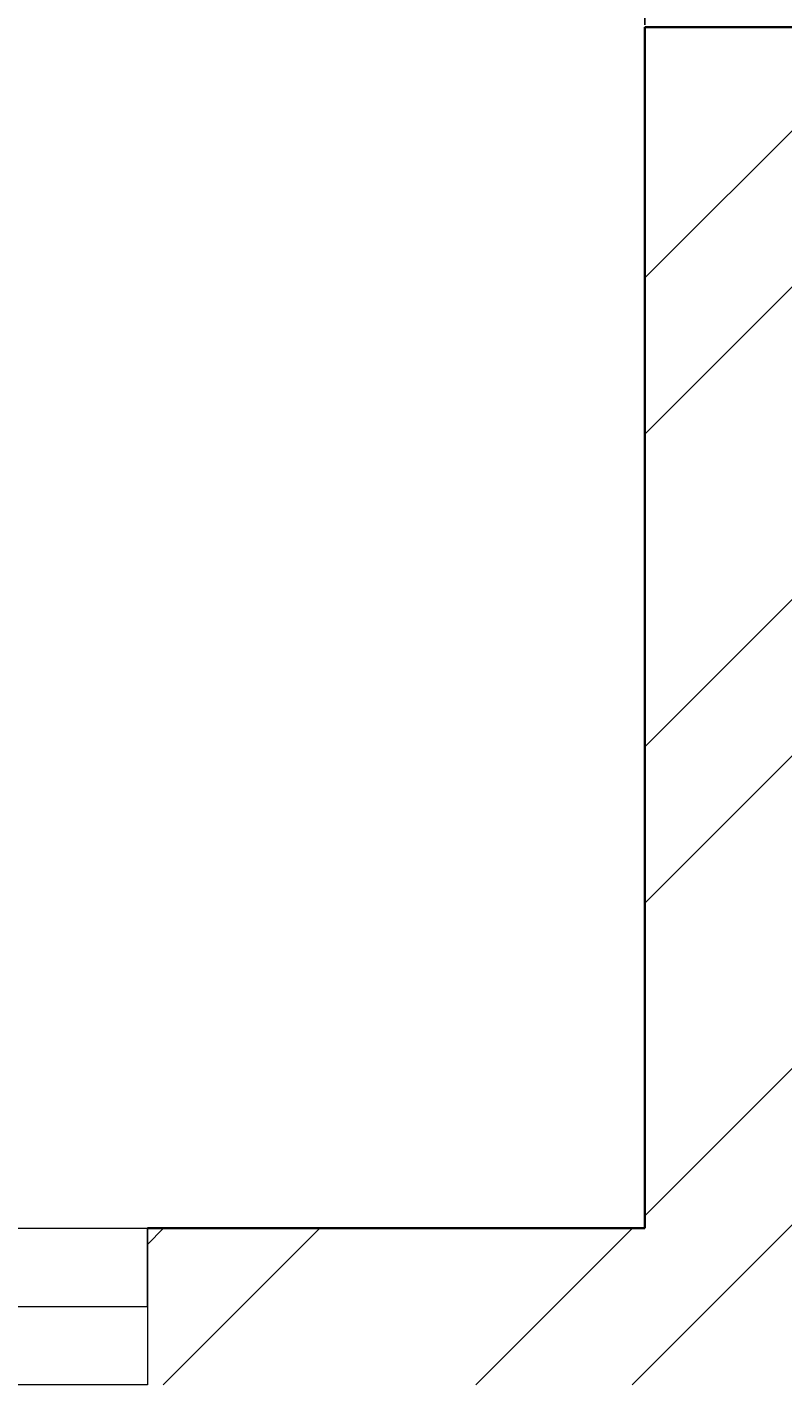
# Model space of a CAD drawing. Units: inches. Extents: x 1885 to 2748, y 783 to 2421.
# Tile 95 of 117: x 2341 to 2363, y 2314 to 2353. Entities that reach past the tile are written whole.
import ezdxf

# ---------------------------------------------------------------- set-up
doc = ezdxf.new("R2010")
doc.units = ezdxf.units.IN
for name, color, linetype, lineweight in [('A-ANNO-DIMS', 2, 'Continuous', 18), ('A-GLAZ', 181, 'Continuous', 18), ('A-WALL', 7, 'Continuous', 35)]:
    doc.layers.add(name, color=color, linetype=linetype, lineweight=lineweight)
doc.layers.add('A-WALL-PATT', color=85, linetype='Continuous', lineweight=13, true_color=0x58ba48)
doc.styles.get("Standard").update_dxf_attribs({"font": 'arial.ttf'})
doc.dimstyles.get("Standard").update_dxf_attribs({"dimtxt": 0.18, "dimasz": 0.18, "dimexe": 0.18, "dimexo": 0.0625, "dimgap": 0.09, "dimtad": 0, "dimtih": 1, "dimtoh": 1, "dimdec": 4, "dimzin": 0, "dimdsep": 46, "dimtxsty": 'Standard', "dimcen": 0.09, "dimadec": 0, "dimazin": 0, "dimtfac": 1, "dimtdec": 4, "dimtofl": 0, "dimtmove": 0, "dimatfit": 3, "dimfxl": 1, "dimtolj": 1, "dimtzin": 0, "dimarcsym": 0})

# ---------------------------------------------------------------- blocks, each defined once
blk = doc.blocks.new('WIN-24')
for p, q in [((0.001, 4.496), (0.001, -0.004)), ((0.001, 4.496), (24.001, 4.496)), ((24.001, 2.246), (24.001, 4.496)), ((24.001, 4.496), (24.001, -0.004)), ((0.001, -0.004), (0.001, 2.246)), ((0.001, 2.246), (24.001, 2.246)), ((24.001, -0.004), (0.001, -0.004))]:
    blk.add_line(p, q)
blk = doc.blocks.new('*D52')
at = {"layer": 'A-ANNO-DIMS', "color": 0, "lineweight": -2, "transparency": 16777216}
for p, q in [((2310.774, 2348.068), (2310.774, 2420.936)), ((2310.954, 2420.756), (2334.551, 2420.756)), ((2358.594, 2420.756), (2334.996, 2420.756)), ((2358.774, 2352.568), (2358.774, 2420.936))]:
    blk.add_line(p, q, dxfattribs=at)
at = {"layer": 'A-ANNO-DIMS', "color": 0, "transparency": 16777216}
for points in [[(2310.954, 2420.786), (2310.954, 2420.726), (2310.774, 2420.756)], [(2358.594, 2420.786), (2358.594, 2420.726), (2358.774, 2420.756)]]:
    blk.add_solid(points, dxfattribs=at)
at = {"layer": 'Defpoints', "color": 0, "transparency": 16777216}
for p in [(2358.774, 2420.756), (2358.774, 2352.506), (2310.774, 2348.006)]:
    blk.add_point(p, dxfattribs=at)
at = {"layer": 'A-ANNO-DIMS', "color": 0, "transparency": 16777216, "insert": (2334.774, 2420.756), "char_height": 0.18, "attachment_point": 5}
blk.add_mtext('\\A1;48', dxfattribs=at)

msp = doc.modelspace()

# ---------------------------------------------------------------- hatches: boundary and pattern name
at = {"layer": 'A-WALL-PATT'}
h = msp.add_hatch(dxfattribs=at)
h.set_pattern_fill('ANSI32', color=256)
h.paths.add_polyline_path([(2007.772, 2318.006), (1980.774, 2318.006), (1980.774, 2281.215), (1985.274, 2281.215), (1985.274, 2313.506), (2007.772, 2313.506), (2007.772, 2315.756)])
h.paths.add_polyline_path([(2094.324, 2318.006), (2067.772, 2318.006), (2067.772, 2313.506), (2094.324, 2313.506), (2094.324, 2315.756)])
h.paths.add_polyline_path([(2131.367, 2315.756), (2131.367, 2318.006), (2131.189, 2318.006), (2112.609, 2318.006), (2112.609, 2313.506), (2117.274, 2313.506), (2117.274, 2255.201), (2121.774, 2255.201), (2121.774, 2313.506), (2131.367, 2313.506)])
h.paths.add_polyline_path([(2190.512, 2318.006), (2155.367, 2318.006), (2155.367, 2313.506), (2169.774, 2313.506), (2169.774, 2229.506), (2121.774, 2229.506), (2121.774, 2233.451), (2119.524, 2233.451), (2117.274, 2233.451), (2117.274, 2201.101), (2121.774, 2201.101), (2121.774, 2225.006), (2169.774, 2225.006), (2169.774, 2165.006), (2306.274, 2165.006), (2306.274, 2066.006), (2310.774, 2066.006), (2344.274, 2066.006), (2486.274, 2066.006), (2486.274, 1886.006), (2483.02, 1886.006), (2483.02, 1881.506), (2486.274, 1881.506), (2486.274, 1880.678), (2490.774, 1880.678), (2490.774, 2070.506), (2344.274, 2070.506), (2310.774, 2070.506), (2310.774, 2165.006), (2310.774, 2173.636), (2308.524, 2173.636), (2306.274, 2173.636), (2306.274, 2169.506), (2174.274, 2169.506), (2174.274, 2313.506), (2190.512, 2313.506), (2190.512, 2315.756)])
h.paths.add_polyline_path([(1985.274, 2221.215), (1980.774, 2221.215), (1980.774, 2165.006), (1992.774, 2165.006), (1992.774, 2141.927), (1997.274, 2141.927), (1997.274, 2165.006), (2117.274, 2165.006), (2117.274, 2163.126), (2121.774, 2163.126), (2121.774, 2172.734), (2119.524, 2172.734), (2117.274, 2172.734), (2117.274, 2169.506), (1985.274, 2169.506)])
h.paths.add_polyline_path([(1997.274, 2105.927), (1992.774, 2105.927), (1992.774, 2070.506), (2016.774, 2070.506), (2016.774, 2059.123), (2019.024, 2059.123), (2021.274, 2059.123), (2021.274, 2070.506), (2117.274, 2070.506), (2117.274, 2022.506), (2114.423, 2022.506), (2114.423, 2018.006), (2123.627, 2018.006), (2123.627, 2020.256), (2123.627, 2022.506), (2121.774, 2022.506), (2121.774, 2142.587), (2119.524, 2142.587), (2117.274, 2142.587), (2117.274, 2075.006), (1997.274, 2075.006)])
h.paths.add_polyline_path([(2092.029, 2020.256), (2092.029, 2022.506), (2021.274, 2022.506), (2021.274, 2035.123), (2016.774, 2035.123), (2016.774, 2018.006), (2016.774, 1978.784), (2021.274, 1978.784), (2021.274, 2018.006), (2092.029, 2018.006)])
h.paths.add_polyline_path([(2260.938, 2022.506), (2153.105, 2022.506), (2153.105, 2020.256), (2153.105, 2018.006), (2155.274, 2018.006), (2155.274, 1886.006), (2107.629, 1886.006), (2107.629, 1881.506), (2182.911, 1881.506), (2182.911, 1883.756), (2182.911, 1886.006), (2159.774, 1886.006), (2159.774, 2018.006), (2260.938, 2018.006), (2260.938, 2020.256)])
h.paths.add_polyline_path([(2047.629, 1883.756), (2047.629, 1886.006), (2021.274, 1886.006), (2021.274, 1918.784), (2019.024, 1918.784), (2016.774, 1918.784), (2016.774, 1881.506), (2047.629, 1881.506)])
h.paths.add_polyline_path([(2306.361, 1883.756), (2306.361, 1886.006), (2296.274, 1886.006), (2296.274, 1982.006), (2316.535, 1982.006), (2316.535, 1984.256), (2316.535, 1986.506), (2296.274, 1986.506), (2296.274, 2022.506), (2289.276, 2022.506), (2289.276, 2018.006), (2291.774, 2018.006), (2291.774, 1886.006), (2242.911, 1886.006), (2242.911, 1881.506), (2306.361, 1881.506)], flags=17)
h.paths.add_polyline_path([(1985.274, 1843.006), (2021.6, 1843.006), (2021.534, 1845.441), (2021.477, 1847.506), (1980.774, 1847.506), (1980.774, 1809.446), (1985.274, 1809.446)])
h.paths.add_polyline_path([(2131.482, 1845.256), (2131.482, 1847.506), (2081.534, 1847.506), (2081.534, 1843.006), (2117.274, 1843.006), (2117.274, 1784.147), (2119.524, 1784.147), (2121.774, 1784.147), (2121.774, 1843.006), (2131.482, 1843.006)])
h.paths.add_polyline_path([(2203.886, 1847.506), (2155.482, 1847.506), (2155.482, 1843.006), (2169.774, 1843.006), (2169.774, 1759.006), (2121.774, 1759.006), (2121.774, 1761.457), (2117.274, 1761.457), (2117.274, 1730.429), (2121.774, 1730.429), (2121.774, 1754.506), (2177.421, 1754.506), (2177.421, 1756.756), (2177.421, 1759.006), (2174.274, 1759.006), (2174.274, 1843.006), (2203.886, 1843.006)])
h.paths.add_polyline_path([(2335.554, 1845.256), (2335.554, 1847.506), (2239.886, 1847.506), (2239.886, 1843.006), (2306.274, 1843.006), (2306.274, 1759.006), (2199.486, 1759.006), (2199.486, 1754.506), (2310.774, 1754.506), (2310.774, 1843.006), (2335.554, 1843.006)])
h.paths.add_polyline_path([(2348.774, 2022.506), (2344.274, 2022.506), (2344.274, 1986.506), (2341.681, 1986.506), (2341.681, 1982.006), (2344.274, 1982.006), (2344.274, 1886.006), (2330.361, 1886.006), (2330.361, 1881.506), (2361.627, 1881.506), (2361.627, 1883.756), (2361.627, 1886.006), (2348.774, 1886.006)], flags=17)
h.paths.add_polyline_path([(2283.251, 2315.756), (2283.251, 2318.006), (2238.512, 2318.006), (2238.512, 2313.506), (2283.251, 2313.506)], flags=17)
h.paths.add_polyline_path([(2363.274, 2348.006), (2388.677, 2348.006), (2388.677, 2350.256), (2388.677, 2352.506), (2358.774, 2352.506), (2358.774, 2348.006), (2358.774, 2318.006), (2344.481, 2318.006), (2344.481, 2313.506), (2358.774, 2313.506), (2358.774, 2229.506), (2310.774, 2229.506), (2310.774, 2231.952), (2306.274, 2231.952), (2306.274, 2205.611), (2310.774, 2205.611), (2310.774, 2225.006), (2358.774, 2225.006), (2358.774, 2211.506), (2452.329, 2211.506), (2452.329, 2213.756), (2452.329, 2216.006), (2363.274, 2216.006), (2363.274, 2318.006)])
h.paths.add_polyline_path([(2310.774, 2313.506), (2320.481, 2313.506), (2320.481, 2315.756), (2320.481, 2318.006), (2302.728, 2318.006), (2302.728, 2313.506), (2306.274, 2313.506), (2306.274, 2251.076), (2310.774, 2251.076)], flags=17)
h.paths.add_polyline_path([(2490.774, 2352.506), (2486.274, 2352.506), (2448.677, 2352.506), (2448.677, 2348.006), (2486.274, 2348.006), (2486.274, 2318.006), (2486.274, 2216.006), (2481.78, 2216.006), (2481.78, 2211.506), (2486.274, 2211.506), (2486.274, 2165.006), (2493.289, 2165.006), (2493.289, 2167.256), (2493.289, 2169.506), (2490.774, 2169.506), (2490.774, 2313.506), (2494.429, 2313.506), (2494.429, 2318.006), (2490.774, 2318.006)])
h.paths.add_polyline_path([(2534.653, 2318.006), (2515.691, 2318.006), (2515.691, 2313.506), (2534.653, 2313.506), (2534.653, 2315.756)])
h.paths.add_polyline_path([(2618.274, 2318.006), (2594.653, 2318.006), (2594.653, 2313.506), (2613.774, 2313.506), (2613.774, 2281.706), (2618.274, 2281.706)])
h.paths.add_polyline_path([(2618.274, 2221.706), (2613.774, 2221.706), (2613.774, 2169.506), (2554.019, 2169.506), (2554.019, 2165.006), (2613.774, 2165.006), (2613.774, 2152.878), (2618.274, 2152.878)])
h.paths.add_polyline_path([(2618.274, 2128.878), (2616.024, 2128.878), (2613.774, 2128.878), (2613.774, 2117.006), (2529.774, 2117.006), (2529.774, 2165.006), (2532.848, 2165.006), (2532.848, 2169.506), (2522.867, 2169.506), (2522.867, 2165.006), (2525.274, 2165.006), (2525.274, 2117.006), (2525.274, 2112.506), (2525.274, 2108.576), (2529.774, 2108.576), (2529.774, 2112.506), (2613.774, 2112.506), (2613.774, 2080.19), (2618.274, 2080.19)])
h.paths.add_polyline_path([(2618.274, 2044.19), (2616.024, 2044.19), (2613.774, 2044.19), (2613.774, 2015.506), (2529.774, 2015.506), (2529.774, 2088.582), (2527.524, 2088.582), (2525.274, 2088.582), (2525.274, 2011.006), (2613.774, 2011.006), (2613.774, 1956.755), (2618.274, 1956.755)])
h.paths.add_polyline_path([(2618.274, 1881.506), (2618.274, 1896.755), (2613.774, 1896.755), (2613.774, 1881.506), (2613.774, 1847.506), (2592.715, 1847.506), (2592.715, 1843.006), (2613.774, 1843.006), (2613.774, 1765.006), (2613.774, 1760.506), (2609.621, 1760.506), (2609.621, 1756.006), (2613.774, 1756.006), (2613.774, 1660.006), (2608.544, 1660.006), (2608.544, 1655.506), (2613.774, 1655.506), (2613.774, 1508.158), (2618.274, 1508.158)])
h.paths.add_polyline_path([(2565.774, 1843.006), (2568.997, 1843.006), (2568.997, 1847.506), (2490.774, 1847.506), (2490.774, 1849.7), (2488.524, 1849.7), (2486.274, 1849.7), (2486.274, 1847.506), (2477.274, 1847.506), (2477.274, 1838.506), (2477.274, 1821.493), (2486.274, 1821.493), (2486.274, 1838.506), (2561.274, 1838.506), (2561.274, 1765.006), (2486.274, 1765.006), (2486.274, 1786.157), (2477.274, 1786.157), (2477.274, 1765.006), (2477.274, 1756.006), (2486.274, 1756.006), (2565.774, 1756.006), (2585.621, 1756.006), (2585.621, 1758.256), (2585.621, 1760.506), (2565.774, 1760.506), (2565.774, 1765.006)])
h.paths.add_polyline_path([(2486.274, 1651.006), (2561.274, 1651.006), (2561.274, 1567.006), (2486.274, 1567.006), (2486.274, 1591.321), (2477.274, 1591.321), (2477.274, 1567.006), (2477.274, 1558.006), (2477.274, 1555.439), (2481.774, 1555.439), (2481.774, 1558.006), (2568.653, 1558.006), (2568.653, 1560.256), (2568.653, 1562.506), (2565.774, 1562.506), (2565.774, 1655.506), (2584.544, 1655.506), (2584.544, 1657.756), (2584.544, 1660.006), (2565.774, 1660.006), (2486.274, 1660.006), (2477.274, 1660.006), (2477.274, 1651.006), (2477.274, 1632.989), (2486.274, 1632.989)])
h.paths.add_polyline_path([(2449.967, 1883.756), (2449.967, 1886.006), (2421.627, 1886.006), (2421.627, 1881.506), (2449.967, 1881.506)], flags=17)
h.paths.add_polyline_path([(2447.274, 1847.506), (2395.554, 1847.506), (2395.554, 1843.006), (2442.774, 1843.006), (2442.774, 1809.27), (2447.274, 1809.27)])
h.paths.add_polyline_path([(1985.274, 1749.446), (1980.774, 1749.446), (1980.774, 1694.504), (1985.274, 1694.504), (1985.274, 1694.506), (1986.897, 1694.506), (1986.897, 1697.78), (1986.897, 1699.006), (1985.274, 1699.006)])
h.paths.add_polyline_path([(2152.774, 1699.006), (2121.774, 1699.006), (2121.774, 1703.668), (2119.524, 1703.668), (2117.274, 1703.668), (2117.274, 1699.006), (2009.219, 1699.006), (2009.219, 1694.506), (2148.274, 1694.506), (2148.274, 1692.631), (2152.774, 1692.631)])
h.paths.add_polyline_path([(2016.274, 1694.506), (2011.774, 1694.506), (2011.774, 1558.006), (2040.806, 1558.006), (2040.806, 1560.256), (2040.806, 1562.506), (2016.274, 1562.506)])
h.paths.add_polyline_path([(2152.774, 1663.017), (2150.524, 1663.017), (2148.274, 1663.017), (2148.274, 1562.506), (2100.806, 1562.506), (2100.806, 1558.006), (2165.119, 1558.006), (2165.119, 1560.256), (2165.119, 1562.506), (2152.774, 1562.506), (2152.774, 1610.506), (2224.774, 1610.506), (2224.774, 1607.99), (2229.274, 1607.99), (2229.274, 1615.006), (2152.774, 1615.006)])
h.paths.add_polyline_path([(2238.613, 1560.256), (2238.613, 1562.506), (2229.274, 1562.506), (2229.274, 1588.756), (2227.024, 1588.763), (2224.774, 1588.771), (2224.774, 1562.506), (2189.119, 1562.506), (2189.119, 1558.006), (2238.613, 1558.006)])
h.paths.add_polyline_path([(2336.024, 1560.256), (2336.024, 1562.506), (2310.774, 1562.506), (2310.774, 1656.347), (2308.524, 1656.347), (2306.274, 1656.347), (2306.274, 1562.506), (2286.613, 1562.506), (2286.613, 1558.006), (2336.024, 1558.006)])
h.paths.add_polyline_path([(2447.274, 1690.968), (2445.024, 1690.968), (2442.774, 1690.968), (2442.774, 1687.006), (2306.274, 1687.006), (2306.274, 1680.75), (2310.774, 1680.75), (2310.774, 1682.506), (2442.774, 1682.506), (2442.774, 1562.506), (2396.024, 1562.506), (2396.024, 1558.006), (2447.274, 1558.006)])
h.paths.add_polyline_path([(2447.274, 1749.27), (2445.024, 1749.27), (2442.774, 1749.27), (2442.774, 1717.232), (2447.274, 1717.232)])
h.paths.add_polyline_path([(2044.674, 1521.756), (2044.674, 1524.006), (2007.274, 1524.006), (2007.274, 1503.49), (2009.524, 1503.49), (2011.774, 1503.49), (2011.774, 1519.506), (2044.674, 1519.506)])
h.paths.add_polyline_path([(2177.969, 1521.756), (2177.969, 1524.006), (2104.674, 1524.006), (2104.674, 1519.506), (2145.774, 1519.506), (2145.774, 1387.506), (2143.37, 1387.506), (2143.37, 1383.006), (2251.585, 1383.006), (2251.585, 1385.256), (2251.585, 1387.506), (2150.274, 1387.506), (2150.274, 1519.506), (2177.969, 1519.506)])
h.paths.add_polyline_path([(2298.704, 1524.006), (2237.969, 1524.006), (2237.969, 1519.506), (2282.274, 1519.506), (2282.274, 1387.506), (2279.683, 1387.506), (2279.683, 1383.006), (2286.774, 1383.006), (2286.774, 1419.006), (2312.451, 1419.006), (2312.451, 1421.256), (2312.451, 1423.506), (2286.774, 1423.506), (2286.774, 1519.506), (2298.704, 1519.506), (2298.704, 1521.722)], flags=17)
h.paths.add_polyline_path([(2361.897, 1521.756), (2361.897, 1524.006), (2322.704, 1524.006), (2322.704, 1519.506), (2334.774, 1519.506), (2334.774, 1423.506), (2331.93, 1423.506), (2331.93, 1419.006), (2334.774, 1419.006), (2334.774, 1387.506), (2334.774, 1383.228), (2339.274, 1383.228), (2339.274, 1387.506), (2339.274, 1519.506), (2361.897, 1519.506)], flags=17)
h.paths.add_polyline_path([(2447.274, 1521.756), (2447.274, 1524.006), (2421.897, 1524.006), (2421.897, 1519.506), (2447.274, 1519.506)], flags=17)
h.paths.add_polyline_path([(2481.774, 1529.6), (2479.524, 1529.6), (2477.274, 1529.6), (2477.274, 1524.006), (2474.489, 1524.006), (2474.489, 1519.506), (2477.274, 1519.506), (2477.274, 1334.506), (2296.774, 1334.506), (2296.774, 1240.506), (2160.274, 1240.506), (2160.274, 1180.506), (2112.274, 1180.506), (2112.274, 1207.692), (2110.024, 1207.692), (2107.774, 1207.692), (2107.774, 1171.609), (2112.274, 1171.609), (2112.274, 1176.006), (2160.274, 1176.006), (2160.274, 1092.006), (2144.221, 1092.006), (2144.221, 1087.506), (2189.497, 1087.506), (2189.497, 1089.756), (2189.497, 1092.006), (2164.774, 1092.006), (2164.774, 1236.006), (2296.774, 1236.006), (2296.774, 1231.912), (2301.274, 1231.912), (2301.274, 1330.006), (2481.774, 1330.006), (2481.774, 1387.506)])
h.paths.add_polyline_path([(2618.274, 1448.158), (2613.774, 1448.158), (2613.774, 1382.506), (2529.774, 1382.506), (2525.274, 1382.506), (2525.274, 1307.062), (2529.774, 1307.062), (2529.774, 1378.006), (2613.774, 1378.006), (2613.774, 1354.988), (2618.274, 1354.988)])
h.paths.add_polyline_path([(2618.274, 1318.988), (2613.774, 1318.988), (2613.774, 1281.006), (2529.774, 1281.006), (2529.774, 1283.786), (2527.524, 1283.786), (2525.274, 1283.786), (2525.274, 1228.506), (2516.794, 1228.506), (2516.794, 1224.006), (2533.484, 1224.006), (2533.484, 1226.256), (2533.484, 1228.506), (2529.774, 1228.506), (2529.774, 1276.506), (2613.774, 1276.506), (2613.774, 1266.02), (2618.274, 1266.02)])
h.paths.add_polyline_path([(2618.274, 1134.964), (2613.774, 1134.964), (2613.774, 1092.006), (2594.545, 1092.006), (2594.545, 1087.506), (2618.274, 1087.506)])
h.paths.add_polyline_path([(2534.545, 1092.006), (2509.765, 1092.006), (2509.765, 1087.506), (2534.545, 1087.506), (2534.545, 1089.756)])
h.paths.add_polyline_path([(2481.274, 1224.006), (2484.117, 1224.006), (2484.117, 1226.256), (2484.117, 1228.506), (2476.774, 1228.506), (2476.774, 1198.506), (2471.61, 1198.506), (2471.61, 1194.006), (2476.774, 1194.006), (2476.774, 1062.006), (2436.894, 1062.006), (2436.894, 1057.506), (2476.774, 1057.506), (2481.274, 1057.506), (2481.274, 1062.006), (2481.274, 1087.506), (2485.354, 1087.506), (2485.354, 1089.756), (2485.354, 1092.006), (2481.274, 1092.006), (2481.274, 1117.506)])
h.paths.add_polyline_path([(2439.898, 1198.506), (2349.274, 1198.506), (2349.274, 1194.006), (2349.274, 1180.506), (2301.274, 1180.506), (2301.274, 1201.896), (2299.024, 1201.896), (2296.774, 1201.896), (2296.774, 1172.335), (2299.024, 1172.335), (2301.274, 1172.335), (2301.274, 1176.006), (2349.274, 1176.006), (2349.274, 1092.006), (2334.452, 1092.006), (2334.452, 1087.506), (2349.274, 1087.506), (2349.274, 1057.506), (2353.774, 1057.506), (2376.894, 1057.506), (2376.894, 1059.756), (2376.894, 1062.006), (2353.774, 1062.006), (2353.774, 1087.506), (2353.774, 1180.506), (2353.774, 1194.006), (2439.898, 1194.006), (2439.898, 1196.256)])
h.paths.add_polyline_path([(2270.596, 1089.756), (2270.596, 1092.006), (2249.497, 1092.006), (2249.497, 1087.506), (2270.596, 1087.506)], flags=17)
h.paths.add_polyline_path([(2310.452, 1092.006), (2301.274, 1092.006), (2301.274, 1153.292), (2296.774, 1153.292), (2296.774, 1092.006), (2293.786, 1092.006), (2293.786, 1087.506), (2310.452, 1087.506), (2310.452, 1089.756)], flags=17)
h.paths.add_polyline_path([(2112.274, 1150.328), (2110.024, 1150.328), (2107.774, 1150.328), (2107.774, 1092.006), (2104.465, 1092.006), (2104.465, 1087.506), (2120.221, 1087.506), (2120.221, 1089.756), (2120.221, 1092.006), (2112.274, 1092.006)])
h.paths.add_polyline_path([(2082.172, 1092.006), (2058.144, 1092.006), (2058.144, 1087.506), (2082.172, 1087.506), (2082.172, 1089.756)])
h.paths.add_polyline_path([(1975.774, 1145.638), (1971.274, 1145.638), (1971.274, 1087.506), (1980.774, 1087.506), (1998.144, 1087.506), (1998.144, 1089.756), (1998.144, 1092.006), (1985.274, 1092.006), (1975.774, 1092.006)])
h.paths.add_polyline_path([(2112.274, 1244.385), (2110.024, 1244.385), (2107.774, 1244.385), (2107.774, 1240.506), (1992.274, 1240.506), (1992.274, 1271.008), (1987.774, 1271.008), (1987.774, 1240.506), (1980.774, 1240.506), (1975.774, 1240.506), (1971.274, 1240.506), (1971.274, 1205.638), (1975.774, 1205.638), (1975.774, 1236.006), (2107.774, 1236.006), (2107.774, 1233.444), (2112.274, 1233.444), (2112.274, 1236.006)])
h.paths.add_polyline_path([(2112.274, 1383.006), (2114.783, 1383.006), (2114.783, 1385.256), (2114.783, 1387.506), (2102.476, 1387.506), (2102.476, 1383.006), (2107.774, 1383.006), (2107.774, 1335.006), (2011.774, 1335.006), (2011.774, 1349.939), (2007.274, 1349.939), (2007.274, 1335.006), (1987.774, 1335.006), (1987.774, 1330.506), (1987.774, 1307.008), (1992.274, 1307.008), (1992.274, 1330.506), (2007.274, 1330.506), (2107.774, 1330.506), (2107.774, 1264.711), (2112.274, 1264.711)])
h.paths.add_polyline_path([(2077.857, 1387.506), (2011.774, 1387.506), (2011.774, 1390.036), (2009.524, 1390.036), (2007.274, 1390.036), (2007.274, 1373.939), (2011.774, 1373.939), (2011.774, 1383.006), (2077.857, 1383.006)])
h.paths.add_polyline_path([(2011.774, 1443.49), (2007.274, 1443.49), (2007.274, 1410.248), (2011.774, 1410.248)])

# ---------------------------------------------------------------- linework, layer by layer
at = {"layer": 'A-WALL'}
for p, q in [((2358.774, 2348.006), (2358.774, 2352.506)), ((2358.774, 2352.506), (2388.677, 2352.506)), ((2358.774, 2318.006), (2358.774, 2348.006)), ((2344.481, 2318.006), (2358.774, 2318.006))]:
    msp.add_line(p, q, dxfattribs=at)

# ---------------------------------------------------------------- block references
at = {"layer": 'A-GLAZ'}
msp.add_blockref('WIN-24', (2320.48, 2313.51), dxfattribs=at)

# ---------------------------------------------------------------- dimensions: what is measured, and where the dimension line sits
at = {"layer": 'A-ANNO-DIMS'}
dim = msp.add_linear_dim(base=(2358.774, 2420.756), p1=(2310.774, 2348.006), p2=(2358.774, 2352.506), dimstyle='Standard', override={"dimdec": 0, "dimlfac": 1, "dimrnd": 0, "dimzin": 0, "dimdsep": 46, "dimlunit": 2}, dxfattribs=at)
dim.commit()
dim.dimension.update_dxf_attribs({"geometry": '*D52', "text_midpoint": (2334.774, 2420.756)})

doc.saveas('drawing.dxf')
